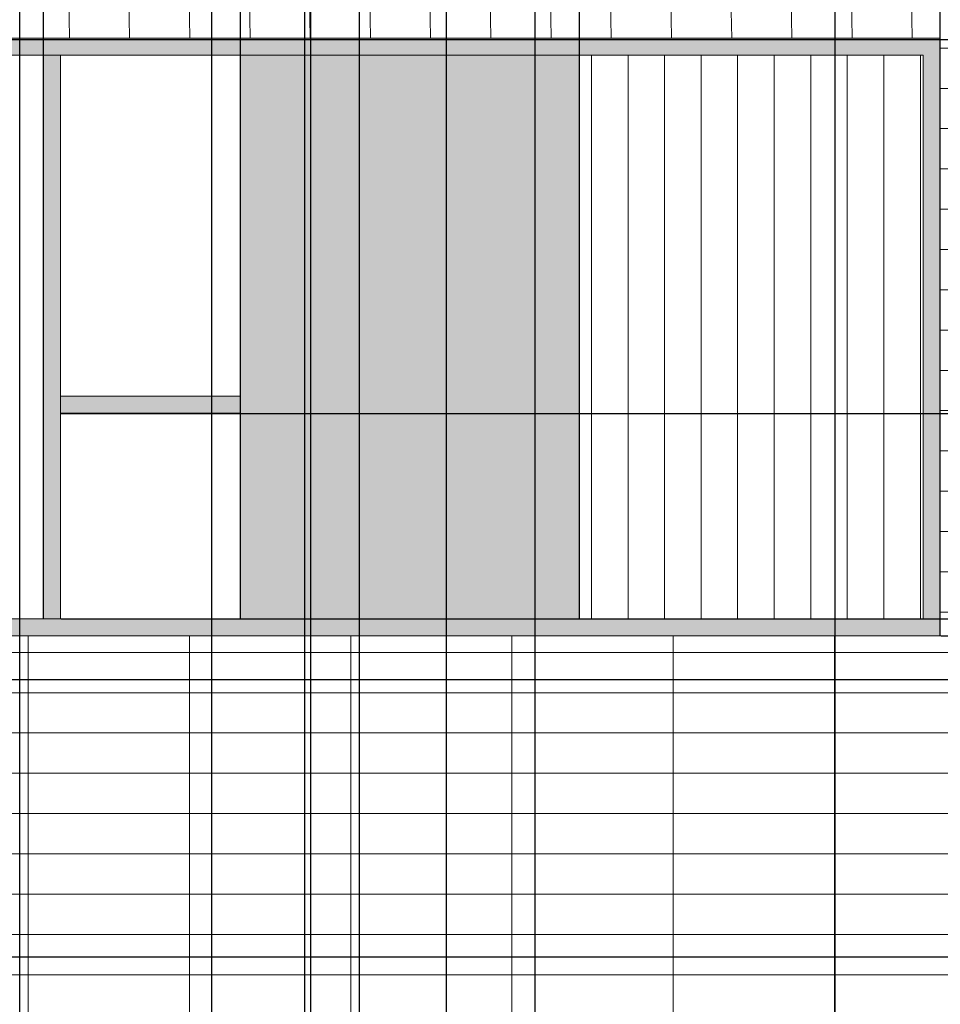
# Model space of a CAD drawing. Units: inches. Extents: x 241 to 943, y 109 to 1396.
# Tile 30 of 34: x 618 to 725, y 1065 to 1180. Entities that reach past the tile are written whole.
import ezdxf

# ---------------------------------------------------------------- set-up
doc = ezdxf.new("R2010")
doc.units = ezdxf.units.IN
doc.header["$MEASUREMENT"] = 0
for name, color, linetype, lineweight in [('A-ANNO-DIMS', 2, 'Continuous', 18), ('A-ELEV', 7, 'Continuous', 25), ('A-ELEV-SHAD', 9, 'Continuous', 13), ('A-GLAZ', 4, 'Continuous', 18), ('A-GLAZ-PATT', 18, 'Continuous', 13), ('A-WALL-PATT', 8, 'Continuous', 13)]:
    doc.layers.add(name, color=color, linetype=linetype, lineweight=lineweight)
doc.styles.get("Standard").update_dxf_attribs({"font": 'arial.ttf'})
doc.dimstyles.get("Standard").update_dxf_attribs({"dimtxt": 1.4375, "dimasz": 0.18, "dimexe": 0.18, "dimexo": 0.0625, "dimgap": 0.09, "dimtad": 0, "dimtih": 1, "dimtoh": 1, "dimdec": 4, "dimzin": 0, "dimdsep": 46, "dimlunit": 4, "dimtxsty": 'Standard', "dimcen": 0.09, "dimadec": 0, "dimazin": 0, "dimtfac": 1, "dimtdec": 4, "dimtofl": 0, "dimtmove": 0, "dimatfit": 3, "dimfxl": 1, "dimtolj": 1, "dimtzin": 0, "dimarcsym": 0})

# ---------------------------------------------------------------- blocks, each defined once
blk = doc.blocks.new('*D12')
at = {"layer": 'A-ANNO-DIMS', "color": 0, "lineweight": -2, "transparency": 16777216}
for p, q in [((530.23, 384.24), (530.23, 1395.05)), ((530.41, 1394.87), (587.56, 1394.87)), ((650.73, 1394.87), (593.58, 1394.87)), ((650.91, 384.24), (650.91, 1395.05))]:
    blk.add_line(p, q, dxfattribs=at)
at = {"layer": 'A-ANNO-DIMS', "color": 0, "transparency": 16777216}
for points in [[(530.41, 1394.9), (530.41, 1394.84), (530.23, 1394.87)], [(650.73, 1394.9), (650.73, 1394.84), (650.91, 1394.87)]]:
    blk.add_solid(points, dxfattribs=at)
at = {"layer": 'Defpoints', "color": 0, "transparency": 16777216}
for p in [(650.91, 1394.87), (530.23, 384.18), (650.91, 384.18)]:
    blk.add_point(p, dxfattribs=at)
at = {"layer": 'A-ANNO-DIMS', "color": 0, "transparency": 16777216, "insert": (590.57, 1394.87), "char_height": 1.438, "attachment_point": 5}
blk.add_mtext('\\A1;120.68', dxfattribs=at)
blk = doc.blocks.new('*D13')
at = {"layer": 'A-ANNO-DIMS', "color": 0, "lineweight": -2, "transparency": 16777216}
for p, q in [((650.91, 384.24), (650.91, 1395.05)), ((651.09, 1394.87), (656.14, 1394.87)), ((667.21, 1394.87), (662.16, 1394.87)), ((667.39, 290.06), (667.39, 1395.05))]:
    blk.add_line(p, q, dxfattribs=at)
at = {"layer": 'A-ANNO-DIMS', "color": 0, "transparency": 16777216}
for points in [[(651.09, 1394.9), (651.09, 1394.84), (650.91, 1394.87)], [(667.21, 1394.9), (667.21, 1394.84), (667.39, 1394.87)]]:
    blk.add_solid(points, dxfattribs=at)
at = {"layer": 'Defpoints', "color": 0, "transparency": 16777216}
for p in [(667.39, 1394.87), (650.91, 384.18), (667.39, 290)]:
    blk.add_point(p, dxfattribs=at)
at = {"layer": 'A-ANNO-DIMS', "color": 0, "transparency": 16777216, "insert": (659.15, 1394.87), "char_height": 1.438, "attachment_point": 5}
blk.add_mtext('\\A1;16.486', dxfattribs=at)
blk = doc.blocks.new('*D14')
at = {"layer": 'A-ANNO-DIMS', "color": 0, "lineweight": -2, "transparency": 16777216}
for p, q in [((667.39, 290.06), (667.39, 1395.05)), ((667.57, 1394.87), (727.7, 1394.87)), ((793.85, 1394.87), (733.72, 1394.87)), ((794.03, 290.06), (794.03, 1395.05))]:
    blk.add_line(p, q, dxfattribs=at)
at = {"layer": 'A-ANNO-DIMS', "color": 0, "transparency": 16777216}
for points in [[(667.57, 1394.9), (667.57, 1394.84), (667.39, 1394.87)], [(793.85, 1394.9), (793.85, 1394.84), (794.03, 1394.87)]]:
    blk.add_solid(points, dxfattribs=at)
at = {"layer": 'Defpoints', "color": 0, "transparency": 16777216}
for p in [(794.03, 1394.87), (667.39, 290), (794.03, 290)]:
    blk.add_point(p, dxfattribs=at)
at = {"layer": 'A-ANNO-DIMS', "color": 0, "transparency": 16777216, "insert": (730.71, 1394.87), "char_height": 1.438, "attachment_point": 5}
blk.add_mtext('\\A1;126.63', dxfattribs=at)
blk = doc.blocks.new('*D49')
at = {"layer": 'A-ANNO-DIMS', "color": 0, "lineweight": -2, "transparency": 16777216}
for p, q in [((766.24, 1177.54), (244.31, 1177.54)), ((244.49, 1177.36), (244.49, 1141.12)), ((244.49, 1103.23), (244.49, 1139.47)), ((766.24, 1103.05), (244.31, 1103.05))]:
    blk.add_line(p, q, dxfattribs=at)
at = {"layer": 'A-ANNO-DIMS', "color": 0, "transparency": 16777216}
for points in [[(244.46, 1177.36), (244.52, 1177.36), (244.49, 1177.54)], [(244.46, 1103.23), (244.52, 1103.23), (244.49, 1103.05)]]:
    blk.add_solid(points, dxfattribs=at)
at = {"layer": 'Defpoints', "color": 0, "transparency": 16777216}
for p in [(244.49, 1177.54), (766.3, 1177.54), (766.3, 1103.05)]:
    blk.add_point(p, dxfattribs=at)
at = {"layer": 'A-ANNO-DIMS', "color": 0, "transparency": 16777216, "insert": (244.49, 1140.29), "char_height": 1.438, "attachment_point": 5}
blk.add_mtext('\\A1;74.49', dxfattribs=at)
blk = doc.blocks.new('*D63')
at = {"layer": 'A-ANNO-DIMS', "color": 0, "lineweight": -2, "transparency": 16777216}
for p, q in [((651.6, 568.89), (651.6, 1395.05)), ((651.78, 1394.87), (719.84, 1394.87)), ((792.51, 1394.87), (724.45, 1394.87)), ((792.69, 568.89), (792.69, 1395.05))]:
    blk.add_line(p, q, dxfattribs=at)
at = {"layer": 'A-ANNO-DIMS', "color": 0, "transparency": 16777216}
for points in [[(651.78, 1394.9), (651.78, 1394.84), (651.6, 1394.87)], [(792.51, 1394.9), (792.51, 1394.84), (792.69, 1394.87)]]:
    blk.add_solid(points, dxfattribs=at)
at = {"layer": 'Defpoints', "color": 0, "transparency": 16777216}
for p in [(792.69, 1394.87), (651.6, 568.83), (792.69, 568.83)]:
    blk.add_point(p, dxfattribs=at)
at = {"layer": 'A-ANNO-DIMS', "color": 0, "transparency": 16777216, "insert": (722.14, 1394.87), "char_height": 1.438, "attachment_point": 5}
blk.add_mtext('\\A1;141.1', dxfattribs=at)
blk = doc.blocks.new('*D66')
at = {"layer": 'A-ANNO-DIMS', "color": 0, "lineweight": -2, "transparency": 16777216}
for p, q in [((617.76, 702.85), (617.76, 1395.05)), ((617.94, 1394.87), (680.69, 1394.87)), ((749.45, 1394.87), (686.7, 1394.87)), ((749.63, 702.85), (749.63, 1395.05))]:
    blk.add_line(p, q, dxfattribs=at)
at = {"layer": 'A-ANNO-DIMS', "color": 0, "transparency": 16777216}
for points in [[(617.94, 1394.9), (617.94, 1394.84), (617.76, 1394.87)], [(749.45, 1394.9), (749.45, 1394.84), (749.63, 1394.87)]]:
    blk.add_solid(points, dxfattribs=at)
at = {"layer": 'Defpoints', "color": 0, "transparency": 16777216}
for p in [(749.63, 1394.87), (617.76, 702.79), (749.63, 702.79)]:
    blk.add_point(p, dxfattribs=at)
at = {"layer": 'A-ANNO-DIMS', "color": 0, "transparency": 16777216, "insert": (683.7, 1394.87), "char_height": 1.438, "attachment_point": 5}
blk.add_mtext('\\A1;131.87', dxfattribs=at)
blk = doc.blocks.new('*D68')
at = {"layer": 'A-ANNO-DIMS', "color": 0, "lineweight": -2, "transparency": 16777216}
for p, q in [((617.76, 841.6), (617.76, 1395.05)), ((617.94, 1394.87), (702.22, 1394.87)), ((792.51, 1394.87), (708.23, 1394.87)), ((792.69, 841.6), (792.69, 1395.05))]:
    blk.add_line(p, q, dxfattribs=at)
at = {"layer": 'A-ANNO-DIMS', "color": 0, "transparency": 16777216}
for points in [[(617.94, 1394.9), (617.94, 1394.84), (617.76, 1394.87)], [(792.51, 1394.9), (792.51, 1394.84), (792.69, 1394.87)]]:
    blk.add_solid(points, dxfattribs=at)
at = {"layer": 'Defpoints', "color": 0, "transparency": 16777216}
for p in [(792.69, 1394.87), (617.76, 841.54), (792.69, 841.54)]:
    blk.add_point(p, dxfattribs=at)
at = {"layer": 'A-ANNO-DIMS', "color": 0, "transparency": 16777216, "insert": (705.23, 1394.87), "char_height": 1.438, "attachment_point": 5}
blk.add_mtext('\\A1;174.93', dxfattribs=at)
blk = doc.blocks.new('*D70')
at = {"layer": 'A-ANNO-DIMS', "color": 0, "lineweight": -2, "transparency": 16777216}
for p, q in [((603.87, 1009.6), (603.87, 1395.05)), ((604.05, 1394.87), (674.69, 1394.87)), ((751.33, 1394.87), (680.69, 1394.87)), ((751.51, 1009.6), (751.51, 1395.05))]:
    blk.add_line(p, q, dxfattribs=at)
at = {"layer": 'A-ANNO-DIMS', "color": 0, "transparency": 16777216}
for points in [[(604.05, 1394.9), (604.05, 1394.84), (603.87, 1394.87)], [(751.33, 1394.9), (751.33, 1394.84), (751.51, 1394.87)]]:
    blk.add_solid(points, dxfattribs=at)
at = {"layer": 'Defpoints', "color": 0, "transparency": 16777216}
for p in [(751.51, 1394.87), (603.87, 1009.54), (751.51, 1009.54)]:
    blk.add_point(p, dxfattribs=at)
at = {"layer": 'A-ANNO-DIMS', "color": 0, "transparency": 16777216, "insert": (677.69, 1394.87), "char_height": 1.438, "attachment_point": 5}
blk.add_mtext('\\A1;147.64', dxfattribs=at)
blk = doc.blocks.new('*D82')
at = {"layer": 'A-ANNO-DIMS', "color": 0, "lineweight": -2, "transparency": 16777216}
for p, q in [((565.2, 568.89), (565.2, 1395.05)), ((565.38, 1394.87), (605.89, 1394.87)), ((651.42, 1394.87), (610.91, 1394.87)), ((651.6, 568.89), (651.6, 1395.05))]:
    blk.add_line(p, q, dxfattribs=at)
at = {"layer": 'A-ANNO-DIMS', "color": 0, "transparency": 16777216}
for points in [[(565.38, 1394.9), (565.38, 1394.84), (565.2, 1394.87)], [(651.42, 1394.9), (651.42, 1394.84), (651.6, 1394.87)]]:
    blk.add_solid(points, dxfattribs=at)
at = {"layer": 'Defpoints', "color": 0, "transparency": 16777216}
for p in [(651.6, 1394.87), (565.2, 568.83), (651.6, 568.83)]:
    blk.add_point(p, dxfattribs=at)
at = {"layer": 'A-ANNO-DIMS', "color": 0, "transparency": 16777216, "insert": (608.4, 1394.87), "char_height": 1.438, "attachment_point": 5}
blk.add_mtext('\\A1;86.40', dxfattribs=at)
blk = doc.blocks.new('*D95')
at = {"layer": 'A-ANNO-DIMS', "color": 0, "lineweight": -2, "transparency": 16777216}
for p, q in [((724.88, 1108.17), (940.6, 1108.17)), ((940.42, 1107.99), (940.42, 1090.34)), ((940.42, 1071.03), (940.42, 1088.69)), ((508.37, 1070.85), (940.6, 1070.85))]:
    blk.add_line(p, q, dxfattribs=at)
at = {"layer": 'A-ANNO-DIMS', "color": 0, "transparency": 16777216}
for points in [[(940.39, 1107.99), (940.45, 1107.99), (940.42, 1108.17)], [(940.39, 1071.03), (940.45, 1071.03), (940.42, 1070.85)]]:
    blk.add_solid(points, dxfattribs=at)
at = {"layer": 'Defpoints', "color": 0, "transparency": 16777216}
for p in [(724.82, 1108.17), (940.42, 1108.17), (508.31, 1070.85)]:
    blk.add_point(p, dxfattribs=at)
at = {"layer": 'A-ANNO-DIMS', "color": 0, "transparency": 16777216, "insert": (940.42, 1089.51), "char_height": 1.438, "attachment_point": 5}
blk.add_mtext('\\A1;37.315', dxfattribs=at)
blk = doc.blocks.new('*D99')
at = {"layer": 'A-ANNO-DIMS', "color": 0, "lineweight": -2, "transparency": 16777216}
for p, q in [((417.09, 181.71), (417.09, 1395.05)), ((417.27, 1394.87), (539.16, 1394.87)), ((667.21, 1394.87), (545.33, 1394.87)), ((667.39, 214.58), (667.39, 1395.05))]:
    blk.add_line(p, q, dxfattribs=at)
at = {"layer": 'A-ANNO-DIMS', "color": 0, "transparency": 16777216}
for points in [[(417.27, 1394.9), (417.27, 1394.84), (417.09, 1394.87)], [(667.21, 1394.9), (667.21, 1394.84), (667.39, 1394.87)]]:
    blk.add_solid(points, dxfattribs=at)
at = {"layer": 'Defpoints', "color": 0, "transparency": 16777216}
for p in [(667.39, 1394.87), (667.39, 214.52), (417.09, 181.65)]:
    blk.add_point(p, dxfattribs=at)
at = {"layer": 'A-ANNO-DIMS', "color": 0, "transparency": 16777216, "insert": (542.24, 1394.87), "char_height": 1.438, "attachment_point": 5}
blk.add_mtext('\\A1;250.30', dxfattribs=at)
blk = doc.blocks.new('*D106')
at = {"layer": 'A-ANNO-DIMS', "color": 0, "lineweight": -2, "transparency": 16777216}
for p, q in [((602.36, 1110.23), (602.36, 1395.05)), ((602.54, 1394.87), (608.99, 1394.87)), ((620.34, 1394.87), (613.89, 1394.87)), ((620.52, 1110.23), (620.52, 1395.05))]:
    blk.add_line(p, q, dxfattribs=at)
at = {"layer": 'A-ANNO-DIMS', "color": 0, "transparency": 16777216}
for points in [[(602.54, 1394.9), (602.54, 1394.84), (602.36, 1394.87)], [(620.34, 1394.9), (620.34, 1394.84), (620.52, 1394.87)]]:
    blk.add_solid(points, dxfattribs=at)
at = {"layer": 'Defpoints', "color": 0, "transparency": 16777216}
for p in [(620.52, 1394.87), (602.36, 1110.17), (620.52, 1110.17)]:
    blk.add_point(p, dxfattribs=at)
at = {"layer": 'A-ANNO-DIMS', "color": 0, "transparency": 16777216, "insert": (611.44, 1394.87), "char_height": 1.438, "attachment_point": 5}
blk.add_mtext('\\A1;18.16', dxfattribs=at)
blk = doc.blocks.new('*D107')
at = {"layer": 'A-ANNO-DIMS', "color": 0, "lineweight": -2, "transparency": 16777216}
for p, q in [((620.52, 1110.23), (620.52, 1395.05)), ((620.7, 1394.87), (628.91, 1394.87)), ((643.27, 1394.87), (635.07, 1394.87)), ((643.45, 1110.23), (643.45, 1395.05))]:
    blk.add_line(p, q, dxfattribs=at)
at = {"layer": 'A-ANNO-DIMS', "color": 0, "transparency": 16777216}
for points in [[(620.7, 1394.9), (620.7, 1394.84), (620.52, 1394.87)], [(643.27, 1394.9), (643.27, 1394.84), (643.45, 1394.87)]]:
    blk.add_solid(points, dxfattribs=at)
at = {"layer": 'Defpoints', "color": 0, "transparency": 16777216}
for p in [(643.45, 1394.87), (620.52, 1110.17), (643.45, 1110.17)]:
    blk.add_point(p, dxfattribs=at)
at = {"layer": 'A-ANNO-DIMS', "color": 0, "transparency": 16777216, "insert": (631.99, 1394.87), "char_height": 1.438, "attachment_point": 5}
blk.add_mtext('\\A1;22.932', dxfattribs=at)
blk = doc.blocks.new('*D108')
at = {"layer": 'A-ANNO-DIMS', "color": 0, "lineweight": -2, "transparency": 16777216}
for p, q in [((643.45, 1110.23), (643.45, 1395.05)), ((643.63, 1394.87), (660.66, 1394.87)), ((682.69, 1394.87), (665.67, 1394.87)), ((682.87, 1110.23), (682.87, 1395.05))]:
    blk.add_line(p, q, dxfattribs=at)
at = {"layer": 'A-ANNO-DIMS', "color": 0, "transparency": 16777216}
for points in [[(643.63, 1394.9), (643.63, 1394.84), (643.45, 1394.87)], [(682.69, 1394.9), (682.69, 1394.84), (682.87, 1394.87)]]:
    blk.add_solid(points, dxfattribs=at)
at = {"layer": 'Defpoints', "color": 0, "transparency": 16777216}
for p in [(682.87, 1394.87), (643.45, 1110.17), (682.87, 1110.17)]:
    blk.add_point(p, dxfattribs=at)
at = {"layer": 'A-ANNO-DIMS', "color": 0, "transparency": 16777216, "insert": (663.16, 1394.87), "char_height": 1.438, "attachment_point": 5}
blk.add_mtext('\\A1;39.42', dxfattribs=at)
blk = doc.blocks.new('*D109')
at = {"layer": 'A-ANNO-DIMS', "color": 0, "lineweight": -2, "transparency": 16777216}
for p, q in [((682.87, 1110.23), (682.87, 1395.05)), ((683.05, 1394.87), (701.31, 1394.87)), ((724.64, 1394.87), (706.39, 1394.87)), ((724.82, 1108.23), (724.82, 1395.05))]:
    blk.add_line(p, q, dxfattribs=at)
at = {"layer": 'A-ANNO-DIMS', "color": 0, "transparency": 16777216}
for points in [[(683.05, 1394.9), (683.05, 1394.84), (682.87, 1394.87)], [(724.64, 1394.9), (724.64, 1394.84), (724.82, 1394.87)]]:
    blk.add_solid(points, dxfattribs=at)
at = {"layer": 'Defpoints', "color": 0, "transparency": 16777216}
for p in [(724.82, 1394.87), (682.87, 1110.17), (724.82, 1108.17)]:
    blk.add_point(p, dxfattribs=at)
at = {"layer": 'A-ANNO-DIMS', "color": 0, "transparency": 16777216, "insert": (703.85, 1394.87), "char_height": 1.438, "attachment_point": 5}
blk.add_mtext('\\A1;41.94', dxfattribs=at)
blk = doc.blocks.new('*D111')
at = {"layer": 'A-ANNO-DIMS', "color": 0, "lineweight": -2, "transparency": 16777216}
for p, q in [((622.58, 1134.07), (940.6, 1134.07)), ((940.42, 1133.89), (940.42, 1122.95)), ((940.42, 1110.35), (940.42, 1121.3)), ((622.58, 1110.17), (940.6, 1110.17))]:
    blk.add_line(p, q, dxfattribs=at)
at = {"layer": 'A-ANNO-DIMS', "color": 0, "transparency": 16777216}
for points in [[(940.39, 1133.89), (940.45, 1133.89), (940.42, 1134.07)], [(940.39, 1110.35), (940.45, 1110.35), (940.42, 1110.17)]]:
    blk.add_solid(points, dxfattribs=at)
at = {"layer": 'Defpoints', "color": 0, "transparency": 16777216}
for p in [(622.52, 1134.07), (940.42, 1134.07), (622.52, 1110.17)]:
    blk.add_point(p, dxfattribs=at)
at = {"layer": 'A-ANNO-DIMS', "color": 0, "transparency": 16777216, "insert": (940.42, 1122.12), "char_height": 1.438, "attachment_point": 5}
blk.add_mtext('\\A1;23.905', dxfattribs=at)
blk = doc.blocks.new('*D113')
at = {"layer": 'A-ANNO-DIMS', "color": 0, "lineweight": -2, "transparency": 16777216}
for p, q in [((603.87, 902.92), (603.87, 1395.05)), ((604.05, 1394.87), (618.91, 1394.87)), ((639.93, 1394.87), (625.07, 1394.87)), ((640.11, 902.92), (640.11, 1395.05))]:
    blk.add_line(p, q, dxfattribs=at)
at = {"layer": 'A-ANNO-DIMS', "color": 0, "transparency": 16777216}
for points in [[(604.05, 1394.9), (604.05, 1394.84), (603.87, 1394.87)], [(639.93, 1394.9), (639.93, 1394.84), (640.11, 1394.87)]]:
    blk.add_solid(points, dxfattribs=at)
at = {"layer": 'Defpoints', "color": 0, "transparency": 16777216}
for p in [(640.11, 1394.87), (603.87, 902.85), (640.11, 902.85)]:
    blk.add_point(p, dxfattribs=at)
at = {"layer": 'A-ANNO-DIMS', "color": 0, "transparency": 16777216, "insert": (621.99, 1394.87), "char_height": 1.438, "attachment_point": 5}
blk.add_mtext('\\A1;36.245', dxfattribs=at)
blk = doc.blocks.new('*D114')
at = {"layer": 'A-ANNO-DIMS', "color": 0, "lineweight": -2, "transparency": 16777216}
for p, q in [((640.11, 902.92), (640.11, 1395.05)), ((640.29, 1394.87), (646.25, 1394.87)), ((657.11, 1394.87), (651.15, 1394.87)), ((657.29, 902.92), (657.29, 1395.05))]:
    blk.add_line(p, q, dxfattribs=at)
at = {"layer": 'A-ANNO-DIMS', "color": 0, "transparency": 16777216}
for points in [[(640.29, 1394.9), (640.29, 1394.84), (640.11, 1394.87)], [(657.11, 1394.9), (657.11, 1394.84), (657.29, 1394.87)]]:
    blk.add_solid(points, dxfattribs=at)
at = {"layer": 'Defpoints', "color": 0, "transparency": 16777216}
for p in [(657.29, 1394.87), (640.11, 902.85), (657.29, 902.85)]:
    blk.add_point(p, dxfattribs=at)
at = {"layer": 'A-ANNO-DIMS', "color": 0, "transparency": 16777216, "insert": (648.7, 1394.87), "char_height": 1.438, "attachment_point": 5}
blk.add_mtext('\\A1;17.18', dxfattribs=at)
blk = doc.blocks.new('*D115')
at = {"layer": 'A-ANNO-DIMS', "color": 0, "lineweight": -2, "transparency": 16777216}
for p, q in [((657.29, 902.92), (657.29, 1395.05)), ((657.47, 1394.87), (664.4, 1394.87)), ((677.51, 1394.87), (670.58, 1394.87)), ((677.69, 902.92), (677.69, 1395.05))]:
    blk.add_line(p, q, dxfattribs=at)
at = {"layer": 'A-ANNO-DIMS', "color": 0, "transparency": 16777216}
for points in [[(657.47, 1394.9), (657.47, 1394.84), (657.29, 1394.87)], [(677.51, 1394.9), (677.51, 1394.84), (677.69, 1394.87)]]:
    blk.add_solid(points, dxfattribs=at)
at = {"layer": 'Defpoints', "color": 0, "transparency": 16777216}
for p in [(677.69, 1394.87), (657.29, 902.85), (677.69, 902.85)]:
    blk.add_point(p, dxfattribs=at)
at = {"layer": 'A-ANNO-DIMS', "color": 0, "transparency": 16777216, "insert": (667.49, 1394.87), "char_height": 1.438, "attachment_point": 5}
blk.add_mtext('\\A1;20.396', dxfattribs=at)
blk = doc.blocks.new('*D116')
at = {"layer": 'A-ANNO-DIMS', "color": 0, "lineweight": -2, "transparency": 16777216}
for p, q in [((677.69, 902.92), (677.69, 1395.05)), ((677.87, 1394.87), (692.06, 1394.87)), ((712.4, 1394.87), (698.22, 1394.87)), ((712.58, 902.92), (712.58, 1395.05))]:
    blk.add_line(p, q, dxfattribs=at)
at = {"layer": 'A-ANNO-DIMS', "color": 0, "transparency": 16777216}
for points in [[(677.87, 1394.9), (677.87, 1394.84), (677.69, 1394.87)], [(712.4, 1394.9), (712.4, 1394.84), (712.58, 1394.87)]]:
    blk.add_solid(points, dxfattribs=at)
at = {"layer": 'Defpoints', "color": 0, "transparency": 16777216}
for p in [(712.58, 1394.87), (677.69, 902.85), (712.58, 902.85)]:
    blk.add_point(p, dxfattribs=at)
at = {"layer": 'A-ANNO-DIMS', "color": 0, "transparency": 16777216, "insert": (695.14, 1394.87), "char_height": 1.438, "attachment_point": 5}
blk.add_mtext('\\A1;34.895', dxfattribs=at)
blk = doc.blocks.new('*D117')
at = {"layer": 'A-ANNO-DIMS', "color": 0, "lineweight": -2, "transparency": 16777216}
for p, q in [((712.58, 902.92), (712.58, 1395.05)), ((712.76, 1394.87), (729.54, 1394.87)), ((751.33, 1394.87), (734.55, 1394.87)), ((751.51, 902.92), (751.51, 1395.05))]:
    blk.add_line(p, q, dxfattribs=at)
at = {"layer": 'A-ANNO-DIMS', "color": 0, "transparency": 16777216}
for points in [[(712.76, 1394.9), (712.76, 1394.84), (712.58, 1394.87)], [(751.33, 1394.9), (751.33, 1394.84), (751.51, 1394.87)]]:
    blk.add_solid(points, dxfattribs=at)
at = {"layer": 'Defpoints', "color": 0, "transparency": 16777216}
for p in [(751.51, 1394.87), (712.58, 902.85), (751.51, 902.85)]:
    blk.add_point(p, dxfattribs=at)
at = {"layer": 'A-ANNO-DIMS', "color": 0, "transparency": 16777216, "insert": (732.05, 1394.87), "char_height": 1.438, "attachment_point": 5}
blk.add_mtext('\\A1;38.92', dxfattribs=at)

msp = doc.modelspace()

# ---------------------------------------------------------------- hatches: boundary and pattern name
at = {"layer": 'A-ELEV-SHAD'}
h = msp.add_hatch(color=256, dxfattribs=at)
h.dxf.hatch_style = 1
h.paths.add_polyline_path([(537.4269, 698.7912), (534.1778, 698.7912), (534.1778, 659.3434), (537.4269, 659.3434)])
h.paths.add_polyline_path([(508.0803, 698.7912), (450.9259, 698.7912), (450.9259, 659.3434), (452.9259, 659.3434), (452.9259, 696.7912), (506.0803, 696.7912), (506.0803, 659.3434), (508.0803, 659.3434)])
h.paths.add_polyline_path([(481.5031, 696.7912), (479.5031, 696.7912), (479.5031, 659.3434), (481.5031, 659.3434)], flags=17)
h.paths.add_polyline_path([(481.5031, 657.3434), (479.5031, 657.3434), (479.5031, 653.3371), (481.5031, 653.3371)], flags=17)
h.paths.add_polyline_path([(508.0803, 657.3434), (506.0803, 657.3434), (506.0803, 653.3371), (452.9259, 653.3371), (452.9259, 657.3434), (450.9259, 657.3434), (450.9259, 651.3371), (508.0803, 651.3371)])
h.paths.add_polyline_path([(428.1173, 839.5382), (426.1173, 839.5382), (426.1173, 786.9154), (428.1173, 786.9154)], flags=17)
h.paths.add_polyline_path([(470.8692, 839.5382), (468.8692, 839.5382), (468.8692, 786.9154), (470.8692, 786.9154)], flags=17)
h.paths.add_polyline_path([(508.3064, 841.5382), (396.3125, 841.5382), (396.3125, 782.5808), (398.3125, 782.5808), (398.3125, 839.5382), (506.3064, 839.5382), (506.3064, 782.5808), (508.3064, 782.5808)])
h.paths.add_polyline_path([(398.3125, 780.5808), (396.3125, 780.5808), (396.3125, 773.4916), (398.3125, 773.4916)])
h.paths.add_polyline_path([(508.3064, 780.5808), (506.3064, 780.5808), (506.3064, 773.4916), (508.3064, 773.4916)])
h.paths.add_polyline_path([(715.6236, 841.5382), (678.2674, 841.5382), (678.2674, 734.8538), (715.6236, 734.8538)])
h.paths.add_polyline_path([(680.2674, 839.5382), (682.4526, 839.5382), (713.6236, 839.5382), (713.6236, 736.9235), (690.2047, 736.9235), (680.2674, 736.9235)], flags=16)
h.paths.add_polyline_path([(792.691, 841.5382), (747.7579, 841.5382), (747.7579, 734.8538), (754.5373, 734.8538), (754.5373, 736.9235), (754.5373, 839.5382), (756.7224, 839.5382), (787.8934, 839.5382), (787.8934, 765.9585), (792.691, 765.9585)])
h.paths.add_polyline_path([(659.2925, 1009.5382), (657.2925, 1009.5382), (657.2925, 902.8538), (659.2925, 902.8538)])
h.paths.add_polyline_path([(751.5078, 976.6275), (712.5839, 976.6275), (712.5839, 974.6275), (751.5078, 974.6275)])
h.paths.add_polyline_path([(470.8692, 1007.5382), (468.8692, 1007.5382), (468.8692, 954.9154), (470.8692, 954.9154)], flags=17)
h.paths.add_polyline_path([(508.3064, 1009.5382), (396.3125, 1009.5382), (396.3125, 950.5808), (398.3125, 950.5808), (398.3125, 1007.5382), (506.3064, 1007.5382), (506.3064, 950.5808), (508.3064, 950.5808)])
h.paths.add_polyline_path([(428.1173, 1007.5382), (426.1173, 1007.5382), (426.1173, 954.9154), (428.1173, 954.9154)], flags=17)
h.paths.add_polyline_path([(398.3125, 948.5808), (396.3125, 948.5808), (396.3125, 941.4916), (398.3125, 941.4916)])
h.paths.add_polyline_path([(508.3064, 948.5808), (506.3064, 948.5808), (506.3064, 941.4916), (508.3064, 941.4916)])
h.paths.add_polyline_path([(428.1173, 1175.5382), (426.1173, 1175.5382), (426.1173, 1122.9154), (428.1173, 1122.9154)], flags=17)
h.paths.add_polyline_path([(508.3064, 1177.5382), (396.3125, 1177.5382), (396.3125, 1118.5808), (398.3125, 1118.5808), (398.3125, 1175.5382), (506.3064, 1175.5382), (506.3064, 1118.5808), (506.8039, 1118.5808, -1), (506.8039, 1116.5808), (506.3064, 1116.5808), (506.3064, 1109.4916), (508.3064, 1109.4916)])
h.paths.add_polyline_path([(470.8692, 1175.5382), (468.8692, 1175.5382), (468.8692, 1122.9154), (470.8692, 1122.9154)], flags=17)
h.paths.add_polyline_path([(398.3125, 1116.5808), (396.3125, 1116.5808), (396.3125, 1109.4916), (398.3125, 1109.4916)], flags=17)
h.paths.add_polyline_path([(724.819, 1177.7336), (533.952, 1177.7336), (533.952, 1108.1686), (724.819, 1108.1686)])
h.paths.add_polyline_path([(535.952, 1175.7336), (722.819, 1175.7336), (722.819, 1110.1686), (535.952, 1110.1686)], flags=0)
h.paths.add_polyline_path([(622.521, 1136.0739), (643.4534, 1136.0739), (643.4534, 1134.0739), (622.521, 1134.0739)], flags=0)
h.paths.add_polyline_path([(722.819, 1175.7336), (535.952, 1175.7336), (535.952, 1110.1686), (722.819, 1110.1686)], flags=16)
h.paths.add_polyline_path([(565.947, 1151.5772), (535.952, 1151.5772), (535.952, 1149.5772), (565.947, 1149.5772)], flags=0)
h = msp.add_hatch(color=256, dxfattribs=at)
h.dxf.hatch_style = 1
h.paths.add_polyline_path([(804.5268, 1142.2929), (768.3038, 1142.2929), (768.3038, 1140.2929), (804.5268, 1140.2929)], flags=0)
h.paths.add_polyline_path([(806.5268, 1177.5382), (766.3038, 1177.5382), (766.3038, 1103.0477), (806.5268, 1103.0477)])
h.paths.add_polyline_path([(768.3038, 1175.5382), (804.5268, 1175.5382), (804.5268, 1105.0477), (768.3038, 1105.0477)], flags=16)
h.paths.add_polyline_path([(643.4534, 1136.0739), (622.521, 1136.0739), (622.521, 1134.0739), (643.4534, 1134.0739)])
h.paths.add_polyline_path([(622.521, 1175.7336), (620.521, 1175.7336), (620.521, 1110.1686), (622.521, 1110.1686)])
h.paths.add_polyline_path([(565.947, 1151.5772), (535.952, 1151.5772), (535.952, 1149.5772), (565.947, 1149.5772)])
at = {"layer": 'A-GLAZ-PATT'}
h = msp.add_hatch(dxfattribs=at)
h.set_pattern_fill('GOST_GLASS', color=256, scale=0.89)
h.set_pattern_definition([(45, (0, 0), (7.5519, 0), [4.45, -6.23]), (45, (1.888, 0), (7.5519, 0), [1.78, -8.9]), (45, (0, 1.888), (7.5519, 0), [1.78, -8.9])])
h.paths.add_polyline_path([(676.8698, 700.7912), (652.0129, 700.7912), (652.0129, 628.4013), (676.8698, 628.4013)])
h.paths.add_polyline_path([(650.0129, 700.7912), (617.7594, 700.7912), (617.7594, 628.4013), (650.0129, 628.4013)])
h.paths.add_polyline_path([(747.7579, 841.5382), (715.6236, 841.5382), (715.6236, 734.8538), (747.7579, 734.8538)])
h.paths.add_polyline_path([(678.2674, 841.5382), (642.9197, 841.5382), (642.9197, 734.8538), (678.2674, 734.8538)])
h.paths.add_polyline_path([(712.5839, 1009.5382), (677.6886, 1009.5382), (677.6886, 902.8538), (712.5839, 902.8538)])
h.paths.add_polyline_path([(640.1141, 1009.5382), (603.8694, 1009.5382), (603.8694, 902.8538), (640.1141, 902.8538)])
h.paths.add_polyline_path([(682.8748, 1175.7336), (643.4534, 1175.7336), (643.4534, 1110.1686), (682.8748, 1110.1686)])
h.paths.add_polyline_path([(602.3616, 1175.7336), (565.947, 1175.7336), (565.947, 1110.1686), (602.3616, 1110.1686)])
h = msp.add_hatch(dxfattribs=at)
h.set_pattern_fill('ANSI31', color=256, scale=34, angle=45)
h.paths.add_polyline_path([(722.819, 1175.7336), (682.8748, 1175.7336), (682.8748, 1110.1686), (722.819, 1110.1686)])
h.paths.add_polyline_path([(642.9197, 841.5382), (617.7594, 841.5382), (617.7594, 734.8538), (642.9197, 734.8538)])
h = msp.add_hatch(dxfattribs=at)
h.set_pattern_fill('ANSI31', color=256, scale=34, angle=45)
h.paths.add_polyline_path([(486.3418, 786.9154), (413.1187, 786.9154), (413.1187, 761.2284), (486.3418, 761.2284)])
h.paths.add_polyline_path([(486.3418, 954.9154), (413.1187, 954.9154), (413.1187, 929.2284), (486.3418, 929.2284)])
h.paths.add_polyline_path([(462.1074, 289.6933), (390.895, 289.6933), (390.895, 277.4626), (390.895, 274.3507), (462.1074, 274.3507), (462.1074, 277.4626)])
h.paths.add_polyline_path([(500.3323, 289.6933), (479.596, 289.6933), (479.596, 274.3507), (500.3323, 274.3507)])
h.paths.add_polyline_path([(450.9259, 566.8295), (426.1086, 566.8295), (426.1086, 498.4395), (446.4348, 498.4395), (446.4348, 519.3754), (450.9259, 519.3754), (450.9259, 525.3816), (445.5808, 525.3816, -1), (445.5808, 527.3816), (450.9259, 527.3816)])
h.paths.add_polyline_path([(563.2023, 508.9074), (534.1778, 508.9074), (508.1906, 508.9074), (508.1906, 498.4395), (563.2023, 498.4395)])
h.paths.add_polyline_path([(747.6328, 700.7912), (712.0171, 700.7912), (712.0171, 628.4013), (747.6328, 628.4013)])
h.paths.add_polyline_path([(446.4348, 643.7483), (426.1086, 643.7483), (426.1086, 630.4013), (446.4348, 630.4013)])
h.paths.add_polyline_path([(564.8076, 841.5382), (553.5166, 841.5382), (508.3064, 841.5382), (508.3064, 782.5808), (564.8076, 782.5808)])
h.paths.add_polyline_path([(564.8076, 780.5808), (508.3064, 780.5808), (508.3064, 773.4916), (564.8076, 773.4916)])
h.paths.add_polyline_path([(792.691, 762.5799), (759.6248, 762.5799), (759.6248, 736.9235), (759.6248, 734.8538), (792.691, 734.8538)])
h.paths.add_polyline_path([(564.8076, 1009.5382), (553.5166, 1009.5382), (508.3064, 1009.5382), (508.3064, 950.5808), (562.3033, 950.5808, -1), (562.3033, 948.5808), (508.3064, 948.5808), (508.3064, 941.4916), (564.8076, 941.4916)])
h.paths.add_polyline_path([(486.3418, 1122.9154), (413.1187, 1122.9154), (413.1187, 1097.2284), (486.3418, 1097.2284)])
at = {"layer": 'A-WALL-PATT'}
h = msp.add_hatch(dxfattribs=at)
h.set_pattern_fill('GRATE', color=256, scale=150)
h.paths.add_polyline_path([(747.7579, 1238.8538), (747.7579, 1275.9142), (747.7579, 1336.1154), (508.3064, 1336.1154), (508.3064, 1275.9142), (508.3064, 1238.8538), (508.3064, 1177.5382), (508.3064, 1109.4916), (508.3064, 1070.8538), (553.5166, 1070.8538), (749.6328, 1070.8538)])
h.paths.add_polyline_path([(533.952, 1108.1686), (533.952, 1177.7336), (533.952, 1303.0286), (724.819, 1303.0286), (724.819, 1108.1686)], flags=16)
h.paths.add_polyline_path([(535.952, 1110.1686), (535.952, 1175.7336), (722.819, 1175.7336), (722.819, 1110.1686)], flags=0)
h.paths.add_polyline_path([(643.4534, 1134.0739), (622.521, 1134.0739), (622.521, 1136.0739), (643.4534, 1136.0739)], flags=0)
h.paths.add_polyline_path([(617.7594, 568.8295), (617.7594, 734.8538), (377.0391, 734.8538), (377.0391, 566.8538), (377.0391, 400.8295), (417.0913, 400.8295), (618.9643, 400.8295)])
h.paths.add_polyline_path([(424.1086, 496.4395), (424.1086, 568.8295), (565.2023, 568.8295), (565.2023, 496.4395)], flags=16)
h.paths.add_polyline_path([(426.1086, 498.4395), (426.1086, 566.8295), (563.2023, 566.8295), (563.2023, 508.9074), (563.2023, 498.4395)], flags=0)
h.paths.add_polyline_path([(508.0803, 508.9074), (508.0803, 519.3754), (450.9259, 519.3754), (450.9259, 525.3816), (445.5808, 525.3816, -1), (445.5808, 527.3816), (450.9259, 527.3816), (450.9259, 566.8295), (508.0803, 566.8295), (537.4269, 566.8295), (537.4269, 508.9074)], flags=0)
h.paths.add_polyline_path([(506.0803, 521.3754), (452.9259, 521.3754), (452.9259, 564.8295), (506.0803, 564.8295)], flags=0)
h.paths.add_polyline_path([(424.1086, 628.4013), (424.1086, 700.7912), (592.9542, 700.7912), (592.9542, 628.4013)], flags=16)
h.paths.add_polyline_path([(426.1086, 630.4013), (426.1086, 698.7912), (590.8792, 698.7912), (590.8792, 630.4013)], flags=0)
h.paths.add_polyline_path([(508.1906, 651.3371), (508.0803, 651.3371), (450.9259, 651.3371), (428.0291, 651.3371), (428.0291, 698.7912), (451.9767, 698.7912), (508.0803, 698.7912), (537.4269, 698.7912), (563.2023, 698.7912), (563.2023, 659.3434), (563.9297, 659.3434), (563.9297, 651.3371)], flags=0)
h.paths.add_polyline_path([(506.0803, 653.3371), (452.9259, 653.3371), (452.9259, 657.3434), (445.5808, 657.3434, -1), (445.5808, 659.3434), (452.9259, 659.3434), (452.9259, 696.7912), (506.0803, 696.7912)], flags=0)
h = msp.add_hatch(dxfattribs=at)
h.set_pattern_fill('ANSI31', color=256, scale=56, angle=46)
h.paths.add_polyline_path([(508.3064, 1275.9142), (377.0391, 1275.9142), (377.0391, 1238.8538), (508.3064, 1238.8538)])
h.paths.add_polyline_path([(724.819, 1237.0695), (533.952, 1237.0695), (533.952, 1177.7336), (724.819, 1177.7336)])
h = msp.add_hatch(dxfattribs=at)
h.set_pattern_fill('GRATE', color=256, scale=150)
h.paths.add_polyline_path([(820.8374, 1070.8538), (749.6328, 1070.8538), (553.5166, 1070.8538), (508.3064, 1070.8538), (508.3064, 1009.5382), (553.5166, 1009.5382), (564.8076, 1009.5382), (603.8694, 1009.5382), (751.5078, 1009.5382), (751.5078, 902.8538), (603.8694, 902.8538), (603.8694, 1009.5382), (564.8076, 1009.5382), (564.8076, 941.4916), (568.1348, 941.4916), (568.1348, 902.8538), (581.3632, 902.8538), (581.3632, 841.5382), (564.8076, 841.5382), (564.8076, 782.5808), (605.9087, 782.5808, -1), (605.9087, 780.5808), (564.8076, 780.5808), (564.8076, 773.4916), (597.514, 773.4916), (607.8162, 773.4916), (607.8162, 734.8538), (617.7594, 734.8538), (617.7594, 841.5382), (792.691, 841.5382), (792.691, 734.8538), (617.7594, 734.8538), (617.7594, 702.7912), (749.6328, 702.7912), (749.6328, 626.4013), (617.7594, 626.4013), (617.7594, 568.8295), (820.8374, 568.8295), (820.8374, 736.8295), (820.8374, 902.8538)])

# ---------------------------------------------------------------- linework, layer by layer
at = {"layer": 'A-ELEV'}
msp.add_line((553.5166, 1070.8538), (749.6328, 1070.8538), dxfattribs=at)
at = {"layer": 'A-GLAZ'}
for p, q in [((620.521, 1175.7336), (620.521, 1110.1686)), ((622.521, 1175.7336), (622.521, 1110.1686)), ((643.4534, 1175.7336), (643.4534, 1110.1686)), ((682.8748, 1175.7336), (682.8748, 1110.1686)), ((622.521, 1136.0739), (643.4534, 1136.0739)), ((622.521, 1134.0739), (643.4534, 1134.0739))]:
    msp.add_line(p, q, dxfattribs=at)
for points in [[(533.952, 1303.0286), (724.819, 1303.0286), (724.819, 1108.1686), (533.952, 1108.1686)], [(533.952, 1177.7336), (724.819, 1177.7336), (724.819, 1108.1686), (533.952, 1108.1686)], [(535.952, 1175.7336), (722.819, 1175.7336), (722.819, 1110.1686), (535.952, 1110.1686)]]:
    msp.add_lwpolyline(points, close=True, dxfattribs=at)

# ---------------------------------------------------------------- dimensions: what is measured, and where the dimension line sits
at = {"layer": 'A-ANNO-DIMS'}
for base, p1, p2, override, picture, middle in [((667.3935, 1394.8654), (417.0913, 181.649), (667.3935, 214.5189), {"dimdec": 2, "dimlfac": 1, "dimrnd": 0, "dimzin": 0, "dimdsep": 46, "dimlunit": 2}, '*D99', (542.2424, 1394.8654)), ((650.907, 1394.8654), (530.2303, 384.1784), (650.907, 384.1784), {"dimdec": 2, "dimlfac": 1, "dimrnd": 0, "dimzin": 0, "dimdsep": 46, "dimlunit": 2}, '*D12', (590.5686, 1394.8654)), ((651.5974, 1394.8654), (565.2023, 568.8295), (651.5974, 568.8295), {"dimdec": 2, "dimlfac": 1, "dimrnd": 0, "dimzin": 0, "dimdsep": 46, "dimlunit": 2}, '*D82', (608.3998, 1394.8654)), ((620.521, 1394.8654), (602.3616, 1110.1686), (620.521, 1110.1686), {"dimdec": 2, "dimlfac": 1, "dimrnd": 0, "dimzin": 0, "dimdsep": 46, "dimlunit": 2}, '*D106', (611.4413, 1394.8654)), ((751.5078, 1394.8654), (603.8694, 1009.5382), (751.5078, 1009.5382), {"dimdec": 2, "dimlfac": 1, "dimrnd": 0, "dimzin": 0, "dimdsep": 46, "dimlunit": 2}, '*D70', (677.6886, 1394.8654)), ((640.1141, 1394.8654), (603.8694, 902.8538), (640.1141, 902.8538), {"dimdec": 3, "dimlfac": 1, "dimrnd": 0, "dimzin": 0, "dimdsep": 46, "dimlunit": 2}, '*D113', (621.9918, 1394.8654)), ((749.6328, 1394.8654), (617.7594, 702.7912), (749.6328, 702.7912), {"dimdec": 2, "dimlfac": 1, "dimrnd": 0, "dimzin": 0, "dimdsep": 46, "dimlunit": 2}, '*D66', (683.6961, 1394.8654)), ((792.691, 1394.8654), (617.7594, 841.5382), (792.691, 841.5382), {"dimdec": 2, "dimlfac": 1, "dimrnd": 0, "dimzin": 0, "dimdsep": 46, "dimlunit": 2}, '*D68', (705.2252, 1394.8654)), ((643.4534, 1394.8654), (620.521, 1110.1686), (643.4534, 1110.1686), {"dimdec": 3, "dimlfac": 1, "dimrnd": 0, "dimzin": 0, "dimdsep": 46, "dimlunit": 2}, '*D107', (631.9872, 1394.8654)), ((657.2925, 1394.8654), (640.1141, 902.8538), (657.2925, 902.8538), {"dimdec": 2, "dimlfac": 1, "dimrnd": 0, "dimzin": 0, "dimdsep": 46, "dimlunit": 2}, '*D114', (648.7033, 1394.8654)), ((682.8748, 1394.8654), (643.4534, 1110.1686), (682.8748, 1110.1686), {"dimdec": 2, "dimlfac": 1, "dimrnd": 0, "dimzin": 0, "dimdsep": 46, "dimlunit": 2}, '*D108', (663.1641, 1394.8654)), ((667.39345, 1394.86544), (650.90697, 384.17836), (667.39345, 289.99842), {"dimdec": 3, "dimlfac": 1, "dimrnd": 0, "dimzin": 0, "dimdsep": 46, "dimlunit": 2}, '*D13', (659.15021, 1394.86544)), ((792.691, 1394.8654), (651.5974, 568.8295), (792.691, 568.8295), {"dimdec": 1, "dimlfac": 1, "dimrnd": 0, "dimzin": 0, "dimdsep": 46, "dimlunit": 2}, '*D63', (722.1442, 1394.8654)), ((677.6886, 1394.8654), (657.2925, 902.8538), (677.6886, 902.8538), {"dimdec": 3, "dimlfac": 1, "dimrnd": 0, "dimzin": 0, "dimdsep": 46, "dimlunit": 2}, '*D115', (667.4905, 1394.8654)), ((794.0275, 1394.8654), (667.3935, 289.9984), (794.0275, 289.9984), {"dimdec": 2, "dimlfac": 1, "dimrnd": 0, "dimzin": 0, "dimdsep": 46, "dimlunit": 2}, '*D14', (730.7105, 1394.8654)), ((712.5839, 1394.8654), (677.6886, 902.8538), (712.5839, 902.8538), {"dimdec": 3, "dimlfac": 1, "dimrnd": 0, "dimzin": 0, "dimdsep": 46, "dimlunit": 2}, '*D116', (695.1363, 1394.8654)), ((724.819, 1394.8654), (682.8748, 1110.1686), (724.819, 1108.1686), {"dimdec": 2, "dimlfac": 1, "dimrnd": 0, "dimzin": 0, "dimdsep": 46, "dimlunit": 2}, '*D109', (703.8469, 1394.8654)), ((751.5078, 1394.8654), (712.5839, 902.8538), (751.5078, 902.8538), {"dimdec": 2, "dimlfac": 1, "dimrnd": 0, "dimzin": 0, "dimdsep": 46, "dimlunit": 2}, '*D117', (732.0459, 1394.8654))]:
    dim = msp.add_linear_dim(base=base, p1=p1, p2=p2, dimstyle='Standard', override=override, dxfattribs=at)
    dim.commit()
    dim.dimension.update_dxf_attribs({"geometry": picture, "text_midpoint": middle})
for base, p1, p2, override, picture, middle in [((244.4858, 1177.5382), (766.3038, 1103.0477), (766.3038, 1177.5382), {"dimdec": 2, "dimlfac": 1, "dimrnd": 0, "dimzin": 0, "dimdsep": 46, "dimlunit": 2}, '*D49', (244.4858, 1140.2929)), ((940.417, 1134.0739), (622.521, 1110.1686), (622.521, 1134.0739), {"dimdec": 3, "dimlfac": 1, "dimrnd": 0, "dimzin": 0, "dimdsep": 46, "dimlunit": 2}, '*D111', (940.417, 1122.1212)), ((940.417, 1108.1686), (508.3064, 1070.8538), (724.819, 1108.1686), {"dimdec": 3, "dimlfac": 1, "dimrnd": 0, "dimzin": 0, "dimdsep": 46, "dimlunit": 2}, '*D95', (940.417, 1089.5112))]:
    dim = msp.add_linear_dim(base=base, p1=p1, p2=p2, angle=90, dimstyle='Standard', override=override, dxfattribs=at)
    dim.commit()
    dim.dimension.update_dxf_attribs({"geometry": picture, "text_midpoint": middle})

doc.saveas('drawing.dxf')
